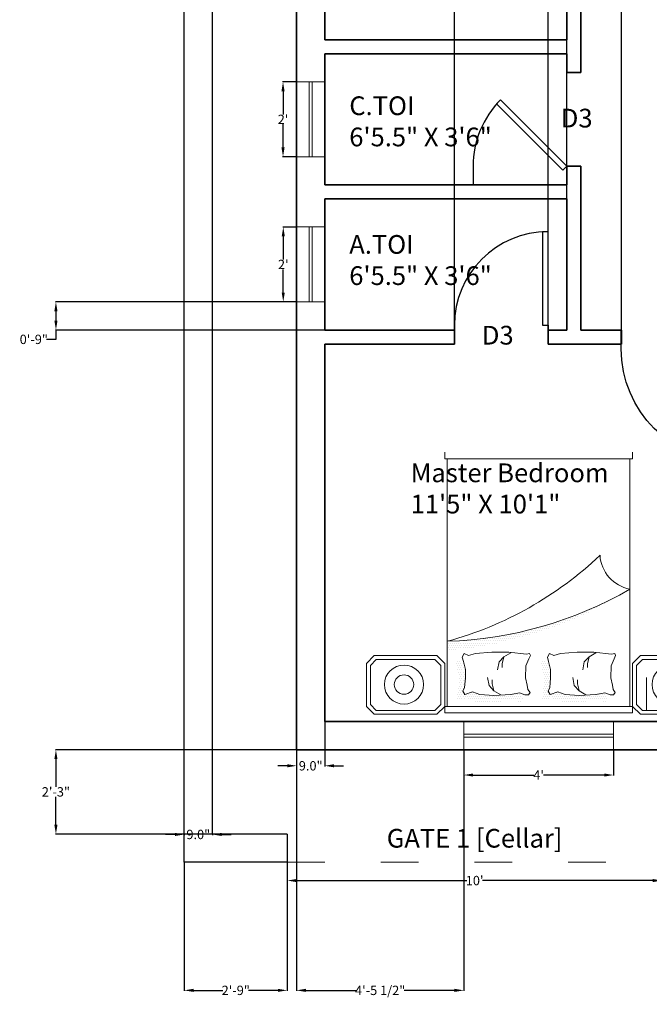
# Model space of a CAD drawing. Units: inches. Extents: x 593 to 1000, y 91 to 964.
# Tile 1 of 4: x 593 to 795, y 91 to 406. Entities that reach past the tile are written whole.
import ezdxf

# ---------------------------------------------------------------- set-up
doc = ezdxf.new("R2010")
doc.units = ezdxf.units.IN
doc.header["$MEASUREMENT"] = 0
doc.linetypes.add('ACAD_ISO03W100', pattern=[30, 12, -18])
for name, color, linetype, lineweight in [('A-ANNO-DIMS', 2, 'Continuous', 13), ('A-ANNO-TEXT', 7, 'Continuous', 18), ('A-AREA-IDEN', 7, 'Continuous', 18), ('A-DOOR', 4, 'Continuous', 25), ('A-GLAZ', 4, 'Continuous', 18), ('A-WALL', 7, 'Continuous', 35), ('C-PROP', 7, 'Continuous', 30), ('C-SITE-GATE', 7, 'ACAD_ISO03W100', 18), ('FUR', 8, 'Continuous', 18)]:
    doc.layers.add(name, color=color, linetype=linetype, lineweight=lineweight)
doc.styles.get("Standard").update_dxf_attribs({"font": 'arial.ttf'})
doc.dimstyles.get("Standard").update_dxf_attribs({"dimtxt": 3, "dimasz": 3, "dimexe": 0.18, "dimexo": 0.0625, "dimgap": 0.09, "dimtad": 0, "dimtih": 1, "dimtoh": 1, "dimdec": 1, "dimzin": 0, "dimdsep": 46, "dimlunit": 3, "dimtxsty": 'Standard', "dimcen": 0.09, "dimadec": 0, "dimazin": 0, "dimtfac": 1, "dimtdec": 1, "dimtofl": 0, "dimtmove": 0, "dimatfit": 3, "dimfxl": 1, "dimtolj": 1, "dimtzin": 0, "dimarcsym": 0})
pattern_1 = [(360, (-204.55691, -125.780183), (0.0079375, 0.015875), [0, -0.015875])]

# ---------------------------------------------------------------- blocks, each defined once
blk = doc.blocks.new('*U4')
for p, q in [((-30, 0), (-30, -6)), ((0, 0), (0, -6))]:
    blk.add_line(p, q)
blk.add_lwpolyline([(0, 0), (-21.21, 21.21), (-22.45, 19.98), (-1.24, -1.24)], close=True)
blk.add_arc((0, 0), 30, 135, 180)
blk = doc.blocks.new('*U6')
for p, q in [((-30, 0), (-30, -6)), ((0, 0), (0, -6))]:
    blk.add_line(p, q)
blk.add_lwpolyline([(0, 0), (0, 30), (-1.75, 30), (-1.75, 0)], close=True)
blk.add_arc((0, 0), 30, 90, 180)
blk = doc.blocks.new('*U5')
for p, q in [((0, 0), (0, 6)), ((36, 0), (36, 6))]:
    blk.add_line(p, q)
blk.add_lwpolyline([(0, 0), (0, -36), (1.75, -36), (1.75, 0)], close=True)
blk.add_arc((0, 0), 36, 270, 0)
blk = doc.blocks.new('A$C9d18b682')
h = blk.add_hatch()
h.set_pattern_fill('DOTS', color=256, scale=0.01, style=0)
h.set_pattern_definition(pattern_1)
h.paths.add_polyline_path([(1.2038, 1.8915), (1.1915, 1.9099), (1.1638, 1.9099), (1.1238, 1.8945), (1.0562, 1.9068), (0.927, 1.916), (0.8193, 1.9068), (0.7639, 1.8884), (0.7055, 1.9068), (0.6901, 1.8822), (0.7024, 1.8546), (0.7086, 1.7839), (0.7086, 1.7163), (0.6932, 1.6548), (0.6839, 1.621), (0.6993, 1.5933), (0.7332, 1.6087), (0.7433, 1.6057), (0.7585, 1.6664), (0.7585, 1.734), (0.7523, 1.8047), (0.74, 1.8324), (0.7554, 1.857), (0.8139, 1.8385), (0.8692, 1.857), (0.9769, 1.8662), (1.1061, 1.857), (1.1738, 1.8447), (1.1846, 1.8488), (1.1884, 1.8699)])
h.paths.add_polyline_path([(1.8571, 1.8915), (1.8448, 1.9099), (1.8171, 1.9099), (1.7771, 1.8945), (1.7095, 1.9068), (1.5803, 1.916), (1.4726, 1.9068), (1.4172, 1.8884), (1.3588, 1.9068), (1.3434, 1.8822), (1.3557, 1.8546), (1.3618, 1.7839), (1.3618, 1.7163), (1.3465, 1.6548), (1.3372, 1.621), (1.3526, 1.5933), (1.3865, 1.6087), (1.3966, 1.6057), (1.4118, 1.6664), (1.4118, 1.734), (1.4056, 1.8047), (1.3933, 1.8324), (1.4087, 1.857), (1.4672, 1.8385), (1.5225, 1.857), (1.6302, 1.8662), (1.7594, 1.857), (1.8271, 1.8447), (1.8379, 1.8488), (1.8417, 1.8699)])
h = blk.add_hatch()
h.set_pattern_fill('DOTS', color=256, scale=0.01, style=0)
h.set_pattern_definition(pattern_1)
h.paths.add_polyline_path([(0.62, 1.5186), (0.62, 1.45, -0.124273), (2.02, 1.05, 0.122563)])
for p, q in [((2.04, 2), (0.6, 2)), ((0.6, 1.95), (0.6, 2)), ((2.04, 2), (2.04, 1.95)), ((2.1476, 1.9789), (2.1476, 1.7289)), ((2.04, 1.95), (0.6, 1.95)), ((0.62, 0.05), (0.62, 1.95)), ((2.02, 1.95), (2.02, 0.05)), ((2.04, 0.05), (0.6, 0.05)), ((0.6, 0), (0.6, 0.05)), ((2.04, 0.05), (2.04, 0))]:
    blk.add_line(p, q)
for points in [[(0.06, 1.56), (0.54, 1.56), (0.6, 1.62), (0.6, 1.95), (0.54, 2.01), (0.06, 2.01), (0, 1.95), (0, 1.62)], [(0.075, 1.59), (0.525, 1.59), (0.57, 1.635), (0.57, 1.935), (0.525, 1.98), (0.075, 1.98), (0.03, 1.935), (0.03, 1.635)], [(2.1, 1.56), (2.58, 1.56), (2.64, 1.62), (2.64, 1.95), (2.58, 2.01), (2.1, 2.01), (2.04, 1.95), (2.04, 1.62)], [(2.115, 1.59), (2.565, 1.59), (2.61, 1.635), (2.61, 1.935), (2.565, 1.98), (2.115, 1.98), (2.07, 1.935), (2.07, 1.635)]]:
    blk.add_lwpolyline(points, close=True)
for points in [[(0.8139, 1.8385), (0.7554, 1.857), (0.74, 1.8324), (0.7523, 1.8047), (0.7585, 1.734), (0.7585, 1.6664), (0.7431, 1.6049), (0.7339, 1.5711), (0.7493, 1.5434), (0.7831, 1.5588), (0.8354, 1.5434), (0.9615, 1.5342), (1.0907, 1.5342), (1.2261, 1.5496), (1.2507, 1.5434), (1.2568, 1.5588), (1.2445, 1.5834), (1.223, 1.6387), (1.2199, 1.7309), (1.2322, 1.7863), (1.2384, 1.8201), (1.2538, 1.8416), (1.2414, 1.86), (1.2138, 1.86), (1.1738, 1.8447), (1.1061, 1.857), (0.9769, 1.8662), (0.8692, 1.857), (0.8139, 1.8385)], [(1.0292, 1.86), (0.9769, 1.8293), (0.94, 1.7893), (0.9277, 1.7279)], [(0.9769, 1.8262), (0.9646, 1.777), (0.9646, 1.7463)], [(1.4672, 1.8385), (1.4087, 1.857), (1.3933, 1.8324), (1.4056, 1.8047), (1.4118, 1.734), (1.4118, 1.6664), (1.3964, 1.6049), (1.3872, 1.5711), (1.4026, 1.5434), (1.4364, 1.5588), (1.4887, 1.5434), (1.6148, 1.5342), (1.744, 1.5342), (1.8794, 1.5496), (1.904, 1.5434), (1.9101, 1.5588), (1.8978, 1.5834), (1.8763, 1.6387), (1.8732, 1.7309), (1.8855, 1.7863), (1.8917, 1.8201), (1.907, 1.8416), (1.8947, 1.86), (1.8671, 1.86), (1.8271, 1.8447), (1.7594, 1.857), (1.6302, 1.8662), (1.5225, 1.857), (1.4672, 1.8385)], [(1.6825, 1.86), (1.6302, 1.8293), (1.5933, 1.7893), (1.581, 1.7279)], [(1.6302, 1.8262), (1.6179, 1.777), (1.6179, 1.7463)], [(1.1061, 1.5373), (1.0538, 1.568), (1.0169, 1.608), (1.0046, 1.6695)], [(1.7594, 1.5373), (1.7071, 1.568), (1.6702, 1.608), (1.6579, 1.6695)], [(1.0538, 1.5711), (1.0415, 1.6203), (1.0415, 1.651)], [(1.7071, 1.5711), (1.6948, 1.6203), (1.6948, 1.651)]]:
    blk.add_lwpolyline(points)
for centre, radius in [((0.288, 1.782), 0.15), ((2.3392, 1.782), 0.15), ((0.288, 1.782), 0.0743), ((2.3392, 1.782), 0.0743)]:
    blk.add_circle(centre, radius)
for centre, radius, start, end in [((0.5277, -1.5229), 2.9743, 59.8866, 88.22261), ((-0.1045, -1.2025), 2.7497, 46.43667, 74.72336), ((2.0704, 0.7742), 0.2804, 100.35432, 176.78617)]:
    blk.add_arc(centre, radius, start, end)
blk = doc.blocks.new('*D15')
at = {"layer": 'A-ANNO-DIMS', "color": 0, "lineweight": -2, "transparency": 16777216}
for p, q in [((678.91, 136.12), (678.91, 130.08)), ((798.91, 136.12), (798.91, 130.08)), ((681.91, 130.26), (736.42, 130.26)), ((795.91, 130.26), (741.4, 130.26))]:
    blk.add_line(p, q, dxfattribs=at)
at = {"layer": 'A-ANNO-DIMS', "color": 0, "transparency": 16777216}
for points in [[(681.91, 130.76), (681.91, 129.76), (678.91, 130.26)], [(795.91, 130.76), (795.91, 129.76), (798.91, 130.26)]]:
    blk.add_solid(points, dxfattribs=at)
at = {"layer": 'Defpoints', "color": 0, "transparency": 16777216}
for p in [(678.91, 136.18), (798.91, 136.18), (798.91, 130.26)]:
    blk.add_point(p, dxfattribs=at)
at = {"layer": 'A-ANNO-DIMS', "color": 0, "transparency": 16777216, "insert": (738.91, 130.26), "char_height": 3, "attachment_point": 5}
blk.add_mtext("\\A1;10'", dxfattribs=at)
blk = doc.blocks.new('*D17')
at = {"layer": 'A-ANNO-DIMS', "color": 0, "lineweight": -2, "transparency": 16777216}
for p, q in [((681.91, 181.12), (681.91, 166.86)), ((690.91, 181.12), (690.91, 166.86)), ((678.91, 167.04), (675.91, 167.04)), ((693.91, 167.04), (696.91, 167.04))]:
    blk.add_line(p, q, dxfattribs=at)
at = {"layer": 'A-ANNO-DIMS', "color": 0, "transparency": 16777216}
for points in [[(678.91, 167.54), (678.91, 166.54), (681.91, 167.04)], [(693.91, 167.54), (693.91, 166.54), (690.91, 167.04)]]:
    blk.add_solid(points, dxfattribs=at)
at = {"layer": 'Defpoints', "color": 0, "transparency": 16777216}
for p in [(681.91, 181.18), (690.91, 181.18), (681.91, 167.04)]:
    blk.add_point(p, dxfattribs=at)
at = {"layer": 'A-ANNO-DIMS', "color": 0, "transparency": 16777216, "insert": (686.41, 167.04), "char_height": 3, "attachment_point": 5}
blk.add_mtext('\\A1;9.0"', dxfattribs=at)
blk = doc.blocks.new('*D19')
at = {"layer": 'A-ANNO-DIMS', "color": 0, "lineweight": -2, "transparency": 16777216}
for p, q in [((681.85, 339.68), (677.44, 339.68)), ((677.62, 336.68), (677.62, 329.28)), ((677.62, 318.68), (677.62, 326.09)), ((681.85, 315.68), (677.44, 315.68))]:
    blk.add_line(p, q, dxfattribs=at)
at = {"layer": 'A-ANNO-DIMS', "color": 0, "transparency": 16777216}
for points in [[(677.12, 336.68), (678.12, 336.68), (677.62, 339.68)], [(677.12, 318.68), (678.12, 318.68), (677.62, 315.68)]]:
    blk.add_solid(points, dxfattribs=at)
at = {"layer": 'Defpoints', "color": 0, "transparency": 16777216}
for p in [(681.91, 339.68), (677.62, 315.68), (681.91, 315.68)]:
    blk.add_point(p, dxfattribs=at)
at = {"layer": 'A-ANNO-DIMS', "color": 0, "transparency": 16777216, "insert": (677.62, 327.68), "char_height": 3, "attachment_point": 5}
blk.add_mtext("\\A1;2'", dxfattribs=at)
blk = doc.blocks.new('*D20')
at = {"layer": 'A-ANNO-DIMS', "color": 0, "lineweight": -2, "transparency": 16777216}
for p, q in [((681.85, 386.18), (677.36, 386.18)), ((677.54, 383.18), (677.54, 375.78)), ((677.54, 365.18), (677.54, 372.59)), ((681.85, 362.18), (677.36, 362.18))]:
    blk.add_line(p, q, dxfattribs=at)
at = {"layer": 'A-ANNO-DIMS', "color": 0, "transparency": 16777216}
for points in [[(677.04, 383.18), (678.04, 383.18), (677.54, 386.18)], [(677.04, 365.18), (678.04, 365.18), (677.54, 362.18)]]:
    blk.add_solid(points, dxfattribs=at)
at = {"layer": 'Defpoints', "color": 0, "transparency": 16777216}
for p in [(681.91, 386.18), (677.54, 362.18), (681.91, 362.18)]:
    blk.add_point(p, dxfattribs=at)
at = {"layer": 'A-ANNO-DIMS', "color": 0, "transparency": 16777216, "insert": (677.54, 374.18), "char_height": 3, "attachment_point": 5}
blk.add_mtext("\\A1;2'", dxfattribs=at)
blk = doc.blocks.new('*D28')
at = {"layer": 'A-ANNO-DIMS', "color": 0, "lineweight": -2, "transparency": 16777216}
for p, q in [((735.41, 172.12), (735.41, 163.9)), ((783.41, 172.12), (783.41, 163.9)), ((738.41, 164.08), (757.88, 164.08)), ((780.41, 164.08), (760.94, 164.08))]:
    blk.add_line(p, q, dxfattribs=at)
at = {"layer": 'A-ANNO-DIMS', "color": 0, "transparency": 16777216}
for points in [[(738.41, 164.58), (738.41, 163.58), (735.41, 164.08)], [(780.41, 164.58), (780.41, 163.58), (783.41, 164.08)]]:
    blk.add_solid(points, dxfattribs=at)
at = {"layer": 'Defpoints', "color": 0, "transparency": 16777216}
for p in [(735.41, 172.18), (783.41, 172.18), (783.41, 164.08)]:
    blk.add_point(p, dxfattribs=at)
at = {"layer": 'A-ANNO-DIMS', "color": 0, "transparency": 16777216, "insert": (759.41, 164.08), "char_height": 3, "attachment_point": 5}
blk.add_mtext("\\A1;4'", dxfattribs=at)
blk = doc.blocks.new('*D35')
at = {"layer": 'A-ANNO-DIMS', "color": 0, "lineweight": -2, "transparency": 16777216}
for p, q in [((642.91, 145.04), (639.91, 145.04)), ((645.91, 145.12), (645.91, 144.86)), ((654.91, 145.12), (654.91, 144.86)), ((657.91, 145.04), (660.91, 145.04))]:
    blk.add_line(p, q, dxfattribs=at)
at = {"layer": 'A-ANNO-DIMS', "color": 0, "transparency": 16777216}
for points in [[(642.91, 145.54), (642.91, 144.54), (645.91, 145.04)], [(657.91, 145.54), (657.91, 144.54), (654.91, 145.04)]]:
    blk.add_solid(points, dxfattribs=at)
at = {"layer": 'Defpoints', "color": 0, "transparency": 16777216}
for p in [(645.91, 145.18), (654.91, 145.18), (645.91, 145.04)]:
    blk.add_point(p, dxfattribs=at)
at = {"layer": 'A-ANNO-DIMS', "color": 0, "transparency": 16777216, "insert": (650.41, 145.04), "char_height": 3, "attachment_point": 5}
blk.add_mtext('\\A1;9.0"', dxfattribs=at)
blk = doc.blocks.new('WIN-24')
for p, q in [((9, 24), (0, 24)), ((4, 24), (4, 0)), ((5, 24), (5, 0)), ((9, 0), (0, 0))]:
    blk.add_line(p, q)
blk = doc.blocks.new('WIN-48')
for p, q in [((0, 0), (0, 9)), ((48, 0), (48, 9)), ((0, 5), (48, 5)), ((0, 4), (48, 4))]:
    blk.add_line(p, q)
blk = doc.blocks.new('*D54')
at = {"layer": 'A-ANNO-DIMS', "color": 0, "lineweight": -2, "transparency": 16777216}
for p, q in [((645.91, 136.12), (645.91, 94.9)), ((678.91, 136.12), (678.91, 94.9)), ((648.91, 95.08), (658.31, 95.08)), ((675.91, 95.08), (666.51, 95.08))]:
    blk.add_line(p, q, dxfattribs=at)
at = {"layer": 'A-ANNO-DIMS', "color": 0, "transparency": 16777216}
for points in [[(648.91, 95.58), (648.91, 94.58), (645.91, 95.08)], [(675.91, 95.58), (675.91, 94.58), (678.91, 95.08)]]:
    blk.add_solid(points, dxfattribs=at)
at = {"layer": 'Defpoints', "color": 0, "transparency": 16777216}
for p in [(645.91, 136.18), (678.91, 136.18), (678.91, 95.08)]:
    blk.add_point(p, dxfattribs=at)
at = {"layer": 'A-ANNO-DIMS', "color": 0, "transparency": 16777216, "insert": (662.41, 95.08), "char_height": 3, "attachment_point": 5}
blk.add_mtext('\\A1;2\'-9"', dxfattribs=at)
blk = doc.blocks.new('*D56')
at = {"layer": 'A-ANNO-DIMS', "color": 0, "lineweight": -2, "transparency": 16777216}
for p, q in [((681.91, 172.12), (681.91, 94.9)), ((735.41, 172.12), (735.41, 94.9)), ((684.91, 95.08), (701.03, 95.08)), ((732.41, 95.08), (716.29, 95.08))]:
    blk.add_line(p, q, dxfattribs=at)
at = {"layer": 'A-ANNO-DIMS', "color": 0, "transparency": 16777216}
for points in [[(684.91, 95.58), (684.91, 94.58), (681.91, 95.08)], [(732.41, 95.58), (732.41, 94.58), (735.41, 95.08)]]:
    blk.add_solid(points, dxfattribs=at)
at = {"layer": 'Defpoints', "color": 0, "transparency": 16777216}
for p in [(681.91, 172.18), (735.41, 172.18), (735.41, 95.08)]:
    blk.add_point(p, dxfattribs=at)
at = {"layer": 'A-ANNO-DIMS', "color": 0, "transparency": 16777216, "insert": (708.66, 95.08), "char_height": 3, "attachment_point": 5}
blk.add_mtext('\\A1;4\'-5 1/2"', dxfattribs=at)
blk = doc.blocks.new('*D57')
at = {"layer": 'A-ANNO-DIMS', "color": 0, "lineweight": -2, "transparency": 16777216}
for p, q in [((681.85, 315.68), (604.63, 315.68)), ((604.81, 312.68), (604.81, 309.68)), ((690.85, 306.68), (604.63, 306.68)), ((604.81, 306.68), (604.81, 303.68)), ((604.81, 303.68), (601.81, 303.68))]:
    blk.add_line(p, q, dxfattribs=at)
at = {"layer": 'A-ANNO-DIMS', "color": 0, "transparency": 16777216}
for points in [[(604.31, 312.68), (605.31, 312.68), (604.81, 315.68)], [(604.31, 309.68), (605.31, 309.68), (604.81, 306.68)]]:
    blk.add_solid(points, dxfattribs=at)
at = {"layer": 'Defpoints', "color": 0, "transparency": 16777216}
for p in [(681.91, 315.68), (604.81, 306.68), (690.91, 306.68)]:
    blk.add_point(p, dxfattribs=at)
at = {"layer": 'A-ANNO-DIMS', "color": 0, "transparency": 16777216, "insert": (597.73, 303.68), "char_height": 3, "attachment_point": 5}
blk.add_mtext('\\A1;0\'-9"', dxfattribs=at)
blk = doc.blocks.new('*D60')
at = {"layer": 'A-ANNO-DIMS', "color": 0, "lineweight": -2, "transparency": 16777216}
for p, q in [((785.91, 306.75), (785.91, 961.96)), ((788.91, 961.78), (799.83, 961.78)), ((818.91, 961.78), (807.99, 961.78)), ((821.91, 306.75), (821.91, 961.96))]:
    blk.add_line(p, q, dxfattribs=at)
at = {"layer": 'A-ANNO-DIMS', "color": 0, "transparency": 16777216}
for points in [[(788.91, 962.28), (788.91, 961.28), (785.91, 961.78)], [(818.91, 962.28), (818.91, 961.28), (821.91, 961.78)]]:
    blk.add_solid(points, dxfattribs=at)
at = {"layer": 'Defpoints', "color": 0, "transparency": 16777216}
for p in [(821.91, 961.78), (785.91, 306.68), (821.91, 306.68)]:
    blk.add_point(p, dxfattribs=at)
at = {"layer": 'A-ANNO-DIMS', "color": 0, "transparency": 16777216, "insert": (803.91, 961.78), "char_height": 3, "attachment_point": 5}
blk.add_mtext('\\A1;3\'-0"', dxfattribs=at)
blk = doc.blocks.new('*D61')
at = {"layer": 'A-ANNO-DIMS', "color": 0, "lineweight": -2, "transparency": 16777216}
for p, q in [((732.41, 306.75), (732.41, 961.96)), ((735.41, 961.78), (743.31, 961.78)), ((759.41, 961.78), (751.51, 961.78)), ((762.41, 306.75), (762.41, 961.96))]:
    blk.add_line(p, q, dxfattribs=at)
at = {"layer": 'A-ANNO-DIMS', "color": 0, "transparency": 16777216}
for points in [[(735.41, 962.28), (735.41, 961.28), (732.41, 961.78)], [(759.41, 962.28), (759.41, 961.28), (762.41, 961.78)]]:
    blk.add_solid(points, dxfattribs=at)
at = {"layer": 'Defpoints', "color": 0, "transparency": 16777216}
for p in [(762.41, 961.78), (732.41, 306.68), (762.41, 306.68)]:
    blk.add_point(p, dxfattribs=at)
at = {"layer": 'A-ANNO-DIMS', "color": 0, "transparency": 16777216, "insert": (747.41, 961.78), "char_height": 3, "attachment_point": 5}
blk.add_mtext('\\A1;2\'-6"', dxfattribs=at)
blk = doc.blocks.new('*D62')
at = {"layer": 'A-ANNO-DIMS', "color": 0, "lineweight": -2, "transparency": 16777216}
for p, q in [((681.85, 172.18), (604.63, 172.18)), ((604.81, 169.18), (604.81, 160.31)), ((604.81, 148.18), (604.81, 157.06)), ((678.85, 145.18), (604.63, 145.18))]:
    blk.add_line(p, q, dxfattribs=at)
at = {"layer": 'A-ANNO-DIMS', "color": 0, "transparency": 16777216}
for points in [[(604.31, 169.18), (605.31, 169.18), (604.81, 172.18)], [(604.31, 148.18), (605.31, 148.18), (604.81, 145.18)]]:
    blk.add_solid(points, dxfattribs=at)
at = {"layer": 'Defpoints', "color": 0, "transparency": 16777216}
for p in [(604.81, 172.18), (681.91, 172.18), (678.91, 145.18)]:
    blk.add_point(p, dxfattribs=at)
at = {"layer": 'A-ANNO-DIMS', "color": 0, "transparency": 16777216, "insert": (604.81, 158.68), "char_height": 3, "attachment_point": 5}
blk.add_mtext('\\A1;2\'-3"', dxfattribs=at)
blk = doc.blocks.new('*D64')
at = {"layer": 'A-ANNO-DIMS', "color": 0, "lineweight": -2, "transparency": 16777216}
for p, q in [((759.41, 961.78), (756.41, 961.78)), ((762.41, 306.75), (762.41, 961.96)), ((768.41, 306.75), (768.41, 961.96)), ((771.41, 961.78), (774.41, 961.78))]:
    blk.add_line(p, q, dxfattribs=at)
at = {"layer": 'A-ANNO-DIMS', "color": 0, "transparency": 16777216}
for points in [[(759.41, 962.28), (759.41, 961.28), (762.41, 961.78)], [(771.41, 962.28), (771.41, 961.28), (768.41, 961.78)]]:
    blk.add_solid(points, dxfattribs=at)
at = {"layer": 'Defpoints', "color": 0, "transparency": 16777216}
for p in [(768.41, 961.78), (762.41, 306.68), (768.41, 306.68)]:
    blk.add_point(p, dxfattribs=at)
at = {"layer": 'A-ANNO-DIMS', "color": 0, "transparency": 16777216, "insert": (778.49, 961.78), "char_height": 3, "attachment_point": 5}
blk.add_mtext('\\A1;0\'-6"', dxfattribs=at)

msp = doc.modelspace()

# ---------------------------------------------------------------- linework, layer by layer
at = {"layer": 'A-WALL'}
for p, q in [((681.91, 172.18), (681.91, 528.23)), ((690.91, 399.68), (690.91, 441.68)), ((768.41, 399.68), (768.41, 441.68)), ((772.91, 399.68), (772.91, 441.68)), ((768.41, 399.68), (690.91, 399.68)), ((772.91, 389.18), (772.91, 399.68)), ((768.41, 395.18), (690.91, 395.18)), ((690.91, 353.18), (690.91, 395.18)), ((768.41, 389.18), (768.41, 395.18)), ((768.41, 389.18), (772.91, 389.18)), ((768.41, 353.18), (768.41, 359.18)), ((768.41, 359.18), (772.91, 359.18)), ((772.91, 353.18), (772.91, 359.18)), ((768.41, 353.18), (690.91, 353.18)), ((772.91, 306.68), (772.91, 353.18)), ((768.41, 348.68), (690.91, 348.68)), ((690.91, 306.68), (690.91, 348.68)), ((768.41, 306.68), (768.41, 348.68)), ((732.41, 306.68), (690.91, 306.68)), ((732.41, 306.68), (732.41, 302.18)), ((762.41, 306.68), (762.41, 302.18)), ((768.41, 306.68), (762.41, 306.68)), ((785.91, 306.68), (772.91, 306.68)), ((785.91, 302.18), (785.91, 306.68)), ((690.91, 181.18), (690.91, 302.18)), ((732.41, 302.18), (690.91, 302.18)), ((785.91, 302.18), (762.41, 302.18)), ((827.91, 181.18), (690.91, 181.18)), ((969.41, 172.18), (681.91, 172.18))]:
    msp.add_line(p, q, dxfattribs=at)
at = {"layer": 'C-PROP'}
msp.add_line((678.91, 145.18), (678.91, 136.18), dxfattribs=at)
for points in [[(678.91, 136.18), (645.91, 136.18), (645.91, 920.68), (978.41, 920.68), (978.41, 136.18), (945.41, 136.18)], [(678.91, 145.18), (654.91, 145.18), (654.91, 911.68), (969.41, 911.68), (969.41, 884.28)]]:
    msp.add_lwpolyline(points, dxfattribs=at)
at = {"layer": 'C-SITE-GATE'}
msp.add_line((678.91, 136.18), (798.91, 136.18), dxfattribs=at)

# ---------------------------------------------------------------- block references
at = {"layer": 'A-DOOR'}
for name, p in [('*U4', (768.41, 359.18)), ('*U6', (762.41, 308.18))]:
    msp.add_blockref(name, p, dxfattribs=at)
at = {"layer": 'A-DOOR', "xscale": -1.001918595307477, "yscale": 1.001918595307477, "zscale": 1.001918595307477}
msp.add_blockref('*U5', (821.91, 300.67), dxfattribs=at)
at = {"layer": 'A-GLAZ'}
for p in [(681.91, 362.19), (681.91, 315.69)]:
    msp.add_blockref('WIN-24', p, dxfattribs=at)
at = {"layer": 'A-GLAZ', "rotation": 180}
msp.add_blockref('WIN-48', (783.41, 181.18), dxfattribs=at)
at = {"layer": 'FUR', "xscale": -41.77713228862137, "yscale": 41.77713228862137, "zscale": 41.77713228862137, "rotation": 179.9999999999977}
msp.add_blockref('A$C9d18b682', (704.26, 267.51), dxfattribs=at)

# ---------------------------------------------------------------- texts
at = {"layer": 'A-ANNO-TEXT', "char_height": 6, "attachment_point": 1}
for s, width, insert in [('{D3}', 8.544, (766.51, 377.57)), ('{D3}', 8.544, (741.23, 308.01)), ('GATE 1 [Cellar]', 76.3054, (710.76, 146.82))]:
    msp.add_mtext_dynamic_manual_height_columns(s, width=width, gutter_width=1, heights=[0], dxfattribs=dict(at, insert=insert))
at = {"layer": 'A-AREA-IDEN', "char_height": 6, "attachment_point": 1}
for s, insert in [('C.TOI\\P6\'5.5" X 3\'6"', (698.76, 381.54)), ('A.TOI\\P6\'5.5" X 3\'6"', (698.76, 337.1)), ('Master Bedroom\\P11\'5" X 10\'1"', (718.43, 263.91))]:
    msp.add_mtext_dynamic_manual_height_columns(s, width=76.3054, gutter_width=1, heights=[0], dxfattribs=dict(at, insert=insert))

# ---------------------------------------------------------------- dimensions: what is measured, and where the dimension line sits
at = {"layer": 'A-ANNO-DIMS'}
for base, p1, p2, override, picture, middle in [((762.41, 961.78), (732.41, 306.68), (762.41, 306.68), {"dimdec": 1, "dimlfac": 1, "dimrnd": 0, "dimzin": 1, "dimdsep": 46, "dimlunit": 4, "dimfrac": 2}, '*D61', (747.41, 961.78)), ((768.41, 961.78), (762.41, 306.68), (768.41, 306.68), {"dimdec": 1, "dimlfac": 1, "dimrnd": 0, "dimzin": 1, "dimdsep": 46, "dimlunit": 4, "dimfrac": 2}, '*D64', (778.49, 961.78)), ((821.91, 961.78), (785.91, 306.68), (821.91, 306.68), {"dimdec": 1, "dimlfac": 1, "dimrnd": 0, "dimzin": 1, "dimdsep": 46, "dimlunit": 4, "dimfrac": 2}, '*D60', (803.91, 961.78)), ((681.91, 167.04), (690.91, 181.18), (681.91, 181.18), {"dimclrd": 0, "dimclre": 0, "dimclrt": 0}, '*D17', (686.41, 167.04)), ((735.41, 95.08), (681.91, 172.18), (735.41, 172.18), {"dimdec": 1, "dimlfac": 1, "dimrnd": 0, "dimzin": 1, "dimdsep": 46, "dimlunit": 4, "dimfrac": 2}, '*D56', (708.66, 95.08)), ((783.41, 164.08), (735.41, 172.18), (783.41, 172.18), {"dimclrd": 0, "dimclre": 0, "dimclrt": 0}, '*D28', (759.41, 164.08)), ((645.91, 145.04), (654.91, 145.18), (645.91, 145.18), {"dimclrd": 0, "dimclre": 0, "dimclrt": 0}, '*D35', (650.41, 145.04)), ((678.91, 95.08), (645.91, 136.18), (678.91, 136.18), {"dimdec": 1, "dimlfac": 1, "dimrnd": 0, "dimzin": 1, "dimdsep": 46, "dimlunit": 4, "dimfrac": 2}, '*D54', (662.41, 95.08)), ((798.91, 130.26), (678.91, 136.18), (798.91, 136.18), {"dimclrd": 0, "dimclre": 0, "dimclrt": 0}, '*D15', (738.91, 130.26))]:
    dim = msp.add_linear_dim(base=base, p1=p1, p2=p2, dimstyle='Standard', override=override, dxfattribs=at)
    dim.commit()
    dim.dimension.update_dxf_attribs({"geometry": picture, "text_midpoint": middle})
for base, p1, p2, override, picture, middle in [((677.54, 362.18), (681.91, 386.18), (681.91, 362.18), {"dimclrd": 0, "dimclre": 0, "dimclrt": 0}, '*D20', (677.54, 374.18)), ((677.62, 315.68), (681.91, 339.68), (681.91, 315.68), {"dimclrd": 0, "dimclre": 0, "dimclrt": 0}, '*D19', (677.62, 327.68)), ((604.81, 306.68), (681.91, 315.68), (690.91, 306.68), {"dimdec": 1, "dimlfac": 1, "dimrnd": 0, "dimzin": 1, "dimdsep": 46, "dimlunit": 4, "dimfrac": 2}, '*D57', (597.73, 303.68)), ((604.81, 172.18), (678.91, 145.18), (681.91, 172.18), {"dimdec": 1, "dimlfac": 1, "dimrnd": 0, "dimzin": 1, "dimdsep": 46, "dimlunit": 4, "dimfrac": 2}, '*D62', (604.81, 158.68))]:
    dim = msp.add_linear_dim(base=base, p1=p1, p2=p2, angle=90, dimstyle='Standard', override=override, dxfattribs=at)
    dim.commit()
    dim.dimension.update_dxf_attribs({"geometry": picture, "text_midpoint": middle})

doc.saveas('drawing.dxf')
